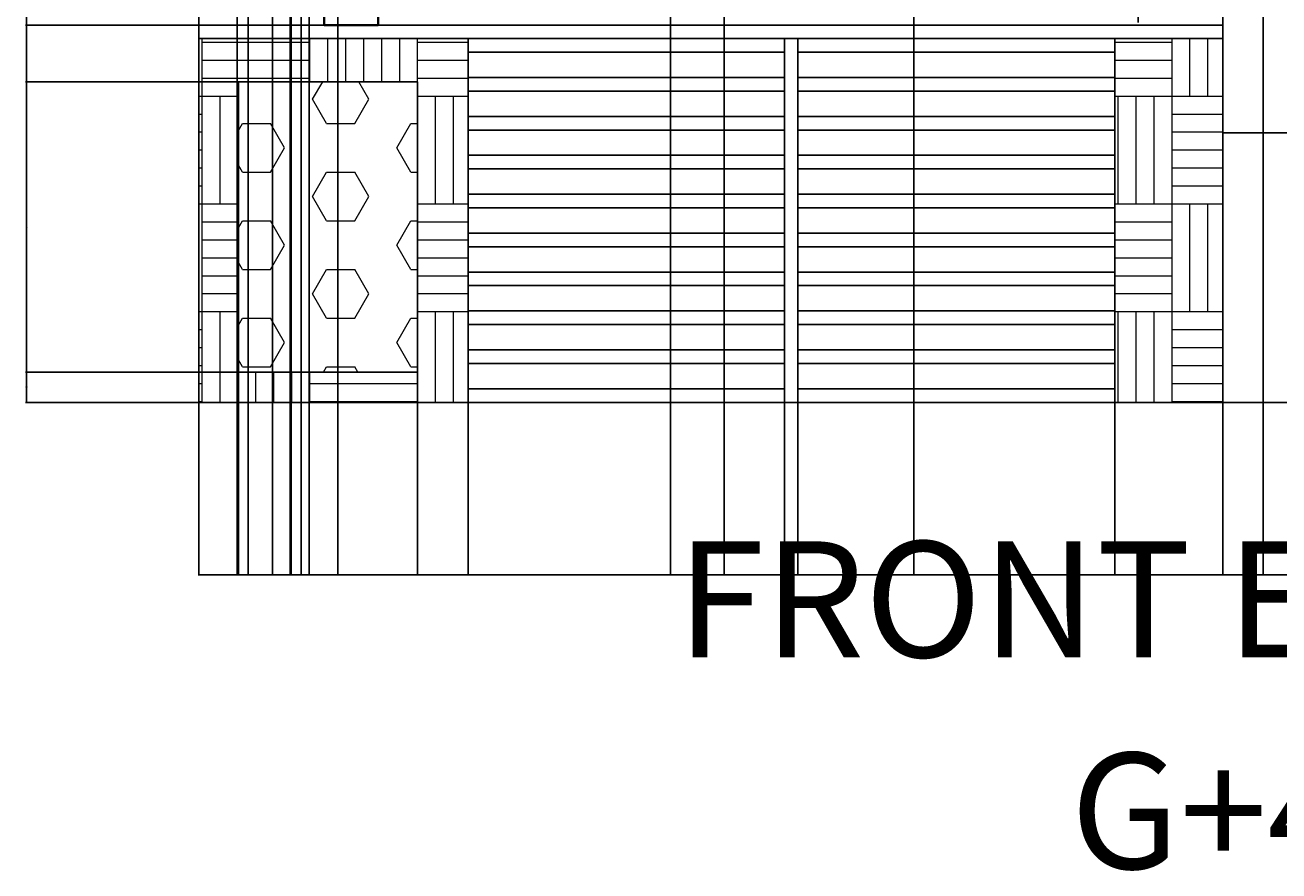
# Model space of a CAD drawing. Units: inches. Extents: x -15 to 605, y -220 to 570.
# Tile 1 of 10: x -15 to 265, y -220 to -32. Entities that reach past the tile are written whole.
import ezdxf

# ---------------------------------------------------------------- set-up
doc = ezdxf.new("R2010")
doc.units = ezdxf.units.IN
doc.header["$MEASUREMENT"] = 0
for name, color, linetype, lineweight in [('A-ANNO-DIMS', 2, 'Continuous', 18), ('A-ANNO-TEXT', 7, 'Continuous', 25), ('A-COLS', 7, 'Continuous', 35), ('A-ELEV-PATT', 8, 'Continuous', 13), ('C-SITE', 3, 'Continuous', 25)]:
    doc.layers.add(name, color=color, linetype=linetype, lineweight=lineweight)
doc.styles.get("Standard").update_dxf_attribs({"font": 'arial.ttf'})
doc.dimstyles.get("Standard").update_dxf_attribs({"dimtxt": 0.18, "dimasz": 0.18, "dimexe": 0.18, "dimexo": 0.0625, "dimgap": 0.09, "dimtad": 0, "dimtih": 1, "dimtoh": 1, "dimdec": 4, "dimzin": 0, "dimdsep": 46, "dimtxsty": 'Standard', "dimcen": 0.09, "dimadec": 0, "dimazin": 0, "dimtfac": 1, "dimtdec": 4, "dimtofl": 0, "dimtmove": 0, "dimatfit": 3, "dimfxl": 1, "dimtolj": 1, "dimtzin": 0, "dimarcsym": 0})

# ---------------------------------------------------------------- blocks, each defined once
blk = doc.blocks.new('*D7')
at = {"layer": 'A-ANNO-DIMS', "color": 0, "lineweight": -2, "transparency": 16777216}
for p, q in [((23.99, 3.76), (23.99, -154.76)), ((566.72, -116.24), (566.72, -154.76)), ((24.17, -154.58), (294.96, -154.58)), ((566.54, -154.58), (295.75, -154.58))]:
    blk.add_line(p, q, dxfattribs=at)
at = {"layer": 'A-ANNO-DIMS', "color": 0, "transparency": 16777216}
for points in [[(24.17, -154.55), (24.17, -154.61), (23.99, -154.58)], [(566.54, -154.55), (566.54, -154.61), (566.72, -154.58)]]:
    blk.add_solid(points, dxfattribs=at)
at = {"layer": 'Defpoints', "color": 0, "transparency": 16777216}
for p in [(23.99, 3.82), (566.72, -116.18), (566.72, -154.58)]:
    blk.add_point(p, dxfattribs=at)
at = {"layer": 'A-ANNO-DIMS', "color": 0, "transparency": 16777216, "insert": (295.35, -154.58), "char_height": 0.18, "attachment_point": 5}
blk.add_mtext('\\A1;542.7', dxfattribs=at)
blk = doc.blocks.new('*D9')
at = {"layer": 'A-ANNO-DIMS', "color": 0, "lineweight": -2, "transparency": 16777216}
for p, q in [((503.92, 531.82), (-14.59, 531.82)), ((-14.41, 531.64), (-14.41, 208)), ((-14.41, -116), (-14.41, 207.64)), ((23.92, -116.18), (-14.59, -116.18))]:
    blk.add_line(p, q, dxfattribs=at)
at = {"layer": 'A-ANNO-DIMS', "color": 0, "transparency": 16777216}
for points in [[(-14.44, 531.64), (-14.38, 531.64), (-14.41, 531.82)], [(-14.44, -116), (-14.38, -116), (-14.41, -116.18)]]:
    blk.add_solid(points, dxfattribs=at)
at = {"layer": 'Defpoints', "color": 0, "transparency": 16777216}
for p in [(-14.41, 531.82), (503.99, 531.82), (23.99, -116.18)]:
    blk.add_point(p, dxfattribs=at)
at = {"layer": 'A-ANNO-DIMS', "color": 0, "transparency": 16777216, "insert": (-14.41, 207.82), "char_height": 0.18, "attachment_point": 5}
blk.add_mtext('\\A1;648', dxfattribs=at)
blk = doc.blocks.new('*D23')
at = {"layer": 'A-ANNO-DIMS', "color": 0, "lineweight": -2, "transparency": 16777216}
for p, q in [((54.93, 15.76), (54.93, -154.76)), ((23.99, 3.76), (23.99, -154.76)), ((24.17, -154.58), (39, -154.58)), ((54.75, -154.58), (39.92, -154.58))]:
    blk.add_line(p, q, dxfattribs=at)
at = {"layer": 'A-ANNO-DIMS', "color": 0, "transparency": 16777216}
for points in [[(24.17, -154.55), (24.17, -154.61), (23.99, -154.58)], [(54.75, -154.55), (54.75, -154.61), (54.93, -154.58)]]:
    blk.add_solid(points, dxfattribs=at)
at = {"layer": 'Defpoints', "color": 0, "transparency": 16777216}
for p in [(54.93, 15.82), (23.99, 3.82), (54.93, -154.58)]:
    blk.add_point(p, dxfattribs=at)
at = {"layer": 'A-ANNO-DIMS', "color": 0, "transparency": 16777216, "insert": (39.46, -154.58), "char_height": 0.18, "attachment_point": 5}
blk.add_mtext('\\A1;30.946', dxfattribs=at)
blk = doc.blocks.new('*D24')
at = {"layer": 'A-ANNO-DIMS', "color": 0, "lineweight": -2, "transparency": 16777216}
for p, q in [((54.93, 15.76), (54.93, -154.76)), ((128.99, 15.76), (128.99, -154.76)), ((55.11, -154.58), (91.57, -154.58)), ((128.81, -154.58), (92.35, -154.58))]:
    blk.add_line(p, q, dxfattribs=at)
at = {"layer": 'A-ANNO-DIMS', "color": 0, "transparency": 16777216}
for points in [[(55.11, -154.55), (55.11, -154.61), (54.93, -154.58)], [(128.81, -154.55), (128.81, -154.61), (128.99, -154.58)]]:
    blk.add_solid(points, dxfattribs=at)
at = {"layer": 'Defpoints', "color": 0, "transparency": 16777216}
for p in [(54.93, 15.82), (128.99, 15.82), (128.99, -154.58)]:
    blk.add_point(p, dxfattribs=at)
at = {"layer": 'A-ANNO-DIMS', "color": 0, "transparency": 16777216, "insert": (91.96, -154.58), "char_height": 0.18, "attachment_point": 5}
blk.add_mtext('\\A1;74.05', dxfattribs=at)
blk = doc.blocks.new('*D25')
at = {"layer": 'A-ANNO-DIMS', "color": 0, "lineweight": -2, "transparency": 16777216}
for p, q in [((128.99, 15.76), (128.99, -154.76)), ((140.99, 15.76), (140.99, -154.76)), ((129.17, -154.58), (134.78, -154.58)), ((140.81, -154.58), (135.2, -154.58))]:
    blk.add_line(p, q, dxfattribs=at)
at = {"layer": 'A-ANNO-DIMS', "color": 0, "transparency": 16777216}
for points in [[(129.17, -154.55), (129.17, -154.61), (128.99, -154.58)], [(140.81, -154.55), (140.81, -154.61), (140.99, -154.58)]]:
    blk.add_solid(points, dxfattribs=at)
at = {"layer": 'Defpoints', "color": 0, "transparency": 16777216}
for p in [(128.99, 15.82), (140.99, 15.82), (140.99, -154.58)]:
    blk.add_point(p, dxfattribs=at)
at = {"layer": 'A-ANNO-DIMS', "color": 0, "transparency": 16777216, "insert": (134.99, -154.58), "char_height": 0.18, "attachment_point": 5}
blk.add_mtext('\\A1;12', dxfattribs=at)
blk = doc.blocks.new('*D26')
at = {"layer": 'A-ANNO-DIMS', "color": 0, "lineweight": -2, "transparency": 16777216}
for p, q in [((140.99, 15.76), (140.99, -154.76)), ((183.17, 15.76), (183.17, -154.76)), ((141.17, -154.58), (161.68, -154.58)), ((182.99, -154.58), (162.48, -154.58))]:
    blk.add_line(p, q, dxfattribs=at)
at = {"layer": 'A-ANNO-DIMS', "color": 0, "transparency": 16777216}
for points in [[(141.17, -154.55), (141.17, -154.61), (140.99, -154.58)], [(182.99, -154.55), (182.99, -154.61), (183.17, -154.58)]]:
    blk.add_solid(points, dxfattribs=at)
at = {"layer": 'Defpoints', "color": 0, "transparency": 16777216}
for p in [(140.99, 15.82), (183.17, 15.82), (183.17, -154.58)]:
    blk.add_point(p, dxfattribs=at)
at = {"layer": 'A-ANNO-DIMS', "color": 0, "transparency": 16777216, "insert": (162.08, -154.58), "char_height": 0.18, "attachment_point": 5}
blk.add_mtext('\\A1;42.18', dxfattribs=at)
blk = doc.blocks.new('*D27')
at = {"layer": 'A-ANNO-DIMS', "color": 0, "lineweight": -2, "transparency": 16777216}
for p, q in [((183.17, 15.76), (183.17, -154.76)), ((260.99, 15.76), (260.99, -154.76)), ((183.35, -154.58), (221.69, -154.58)), ((260.81, -154.58), (222.47, -154.58))]:
    blk.add_line(p, q, dxfattribs=at)
at = {"layer": 'A-ANNO-DIMS', "color": 0, "transparency": 16777216}
for points in [[(183.35, -154.55), (183.35, -154.61), (183.17, -154.58)], [(260.81, -154.55), (260.81, -154.61), (260.99, -154.58)]]:
    blk.add_solid(points, dxfattribs=at)
at = {"layer": 'Defpoints', "color": 0, "transparency": 16777216}
for p in [(183.17, 15.82), (260.99, 15.82), (260.99, -154.58)]:
    blk.add_point(p, dxfattribs=at)
at = {"layer": 'A-ANNO-DIMS', "color": 0, "transparency": 16777216, "insert": (222.08, -154.58), "char_height": 0.18, "attachment_point": 5}
blk.add_mtext('\\A1;77.82', dxfattribs=at)
blk = doc.blocks.new('*D28')
at = {"layer": 'A-ANNO-DIMS', "color": 0, "lineweight": -2, "transparency": 16777216}
for p, q in [((260.99, 15.76), (260.99, -154.76)), ((272.99, 15.76), (272.99, -154.76)), ((261.17, -154.58), (266.78, -154.58)), ((272.81, -154.58), (267.2, -154.58))]:
    blk.add_line(p, q, dxfattribs=at)
at = {"layer": 'A-ANNO-DIMS', "color": 0, "transparency": 16777216}
for points in [[(261.17, -154.55), (261.17, -154.61), (260.99, -154.58)], [(272.81, -154.55), (272.81, -154.61), (272.99, -154.58)]]:
    blk.add_solid(points, dxfattribs=at)
at = {"layer": 'Defpoints', "color": 0, "transparency": 16777216}
for p in [(260.99, 15.82), (272.99, 15.82), (272.99, -154.58)]:
    blk.add_point(p, dxfattribs=at)
at = {"layer": 'A-ANNO-DIMS', "color": 0, "transparency": 16777216, "insert": (266.99, -154.58), "char_height": 0.18, "attachment_point": 5}
blk.add_mtext('\\A1;12', dxfattribs=at)
blk = doc.blocks.new('*D39')
at = {"layer": 'A-ANNO-DIMS', "color": 0, "lineweight": -2, "transparency": 16777216}
for p, q in [((32.79, -109.51), (32.79, -154.76)), ((23.99, -116.24), (23.99, -154.76)), ((24.17, -154.58), (28.01, -154.58)), ((32.61, -154.58), (28.76, -154.58))]:
    blk.add_line(p, q, dxfattribs=at)
at = {"layer": 'A-ANNO-DIMS', "color": 0, "transparency": 16777216}
for points in [[(24.17, -154.55), (24.17, -154.61), (23.99, -154.58)], [(32.61, -154.55), (32.61, -154.61), (32.79, -154.58)]]:
    blk.add_solid(points, dxfattribs=at)
at = {"layer": 'Defpoints', "color": 0, "transparency": 16777216}
for p in [(32.79, -109.45), (23.99, -116.18), (32.79, -154.58)]:
    blk.add_point(p, dxfattribs=at)
at = {"layer": 'A-ANNO-DIMS', "color": 0, "transparency": 16777216, "insert": (28.39, -154.58), "char_height": 0.18, "attachment_point": 5}
blk.add_mtext('\\A1;8.801', dxfattribs=at)
blk = doc.blocks.new('*D40')
at = {"layer": 'A-ANNO-DIMS', "color": 0, "lineweight": -2, "transparency": 16777216}
for p, q in [((32.79, -109.51), (32.79, -154.76)), ((72.68, -109.51), (72.68, -154.76)), ((32.97, -154.58), (52.27, -154.58)), ((72.5, -154.58), (53.2, -154.58))]:
    blk.add_line(p, q, dxfattribs=at)
at = {"layer": 'A-ANNO-DIMS', "color": 0, "transparency": 16777216}
for points in [[(32.97, -154.55), (32.97, -154.61), (32.79, -154.58)], [(72.5, -154.55), (72.5, -154.61), (72.68, -154.58)]]:
    blk.add_solid(points, dxfattribs=at)
at = {"layer": 'Defpoints', "color": 0, "transparency": 16777216}
for p in [(32.79, -109.45), (72.68, -109.45), (72.68, -154.58)]:
    blk.add_point(p, dxfattribs=at)
at = {"layer": 'A-ANNO-DIMS', "color": 0, "transparency": 16777216, "insert": (52.74, -154.58), "char_height": 0.18, "attachment_point": 5}
blk.add_mtext('\\A1;39.895', dxfattribs=at)
blk = doc.blocks.new('*D41')
at = {"layer": 'A-ANNO-DIMS', "color": 0, "lineweight": -2, "transparency": 16777216}
for p, q in [((72.68, -109.51), (72.68, -154.76)), ((83.99, -116.24), (83.99, -154.76)), ((72.86, -154.58), (77.88, -154.58)), ((83.81, -154.58), (78.79, -154.58))]:
    blk.add_line(p, q, dxfattribs=at)
at = {"layer": 'A-ANNO-DIMS', "color": 0, "transparency": 16777216}
for points in [[(72.86, -154.55), (72.86, -154.61), (72.68, -154.58)], [(83.81, -154.55), (83.81, -154.61), (83.99, -154.58)]]:
    blk.add_solid(points, dxfattribs=at)
at = {"layer": 'Defpoints', "color": 0, "transparency": 16777216}
for p in [(72.68, -109.45), (83.99, -116.18), (83.99, -154.58)]:
    blk.add_point(p, dxfattribs=at)
at = {"layer": 'A-ANNO-DIMS', "color": 0, "transparency": 16777216, "insert": (78.34, -154.58), "char_height": 0.18, "attachment_point": 5}
blk.add_mtext('\\A1;11.303', dxfattribs=at)
blk = doc.blocks.new('*D42')
at = {"layer": 'A-ANNO-DIMS', "color": 0, "lineweight": -2, "transparency": 16777216}
for p, q in [((83.99, -116.24), (83.99, -154.76)), ((154.43, -116.24), (154.43, -154.76)), ((84.17, -154.58), (118.82, -154.58)), ((154.25, -154.58), (119.6, -154.58))]:
    blk.add_line(p, q, dxfattribs=at)
at = {"layer": 'A-ANNO-DIMS', "color": 0, "transparency": 16777216}
for points in [[(84.17, -154.55), (84.17, -154.61), (83.99, -154.58)], [(154.25, -154.55), (154.25, -154.61), (154.43, -154.58)]]:
    blk.add_solid(points, dxfattribs=at)
at = {"layer": 'Defpoints', "color": 0, "transparency": 16777216}
for p in [(83.99, -116.18), (154.43, -116.18), (154.43, -154.58)]:
    blk.add_point(p, dxfattribs=at)
at = {"layer": 'A-ANNO-DIMS', "color": 0, "transparency": 16777216, "insert": (119.21, -154.58), "char_height": 0.18, "attachment_point": 5}
blk.add_mtext('\\A1;70.45', dxfattribs=at)
blk = doc.blocks.new('*D43')
at = {"layer": 'A-ANNO-DIMS', "color": 0, "lineweight": -2, "transparency": 16777216}
for p, q in [((154.43, -116.24), (154.43, -154.76)), ((157.4, -116.24), (157.4, -154.76)), ((154.61, -154.58), (155.52, -154.58)), ((157.22, -154.58), (156.31, -154.58))]:
    blk.add_line(p, q, dxfattribs=at)
at = {"layer": 'A-ANNO-DIMS', "color": 0, "transparency": 16777216}
for points in [[(154.61, -154.55), (154.61, -154.61), (154.43, -154.58)], [(157.22, -154.55), (157.22, -154.61), (157.4, -154.58)]]:
    blk.add_solid(points, dxfattribs=at)
at = {"layer": 'Defpoints', "color": 0, "transparency": 16777216}
for p in [(154.43, -116.18), (157.4, -116.18), (157.4, -154.58)]:
    blk.add_point(p, dxfattribs=at)
at = {"layer": 'A-ANNO-DIMS', "color": 0, "transparency": 16777216, "insert": (155.92, -154.58), "char_height": 0.18, "attachment_point": 5}
blk.add_mtext('\\A1;2.969', dxfattribs=at)
blk = doc.blocks.new('*D44')
at = {"layer": 'A-ANNO-DIMS', "color": 0, "lineweight": -2, "transparency": 16777216}
for p, q in [((157.4, -116.24), (157.4, -154.76)), ((227.99, -116.24), (227.99, -154.76)), ((157.58, -154.58), (192.3, -154.58)), ((227.81, -154.58), (193.09, -154.58))]:
    blk.add_line(p, q, dxfattribs=at)
at = {"layer": 'A-ANNO-DIMS', "color": 0, "transparency": 16777216}
for points in [[(157.58, -154.55), (157.58, -154.61), (157.4, -154.58)], [(227.81, -154.55), (227.81, -154.61), (227.99, -154.58)]]:
    blk.add_solid(points, dxfattribs=at)
at = {"layer": 'Defpoints', "color": 0, "transparency": 16777216}
for p in [(157.4, -116.18), (227.99, -116.18), (227.99, -154.58)]:
    blk.add_point(p, dxfattribs=at)
at = {"layer": 'A-ANNO-DIMS', "color": 0, "transparency": 16777216, "insert": (192.69, -154.58), "char_height": 0.18, "attachment_point": 5}
blk.add_mtext('\\A1;70.59', dxfattribs=at)
blk = doc.blocks.new('*D45')
at = {"layer": 'A-ANNO-DIMS', "color": 0, "lineweight": -2, "transparency": 16777216}
for p, q in [((227.99, -116.24), (227.99, -154.76)), ((251.99, -116.24), (251.99, -154.76)), ((228.17, -154.58), (239.77, -154.58)), ((251.81, -154.58), (240.21, -154.58))]:
    blk.add_line(p, q, dxfattribs=at)
at = {"layer": 'A-ANNO-DIMS', "color": 0, "transparency": 16777216}
for points in [[(228.17, -154.55), (228.17, -154.61), (227.99, -154.58)], [(251.81, -154.55), (251.81, -154.61), (251.99, -154.58)]]:
    blk.add_solid(points, dxfattribs=at)
at = {"layer": 'Defpoints', "color": 0, "transparency": 16777216}
for p in [(227.99, -116.18), (251.99, -116.18), (251.99, -154.58)]:
    blk.add_point(p, dxfattribs=at)
at = {"layer": 'A-ANNO-DIMS', "color": 0, "transparency": 16777216, "insert": (239.99, -154.58), "char_height": 0.18, "attachment_point": 5}
blk.add_mtext('\\A1;24', dxfattribs=at)
blk = doc.blocks.new('*D46')
at = {"layer": 'A-ANNO-DIMS', "color": 0, "lineweight": -2, "transparency": 16777216}
for p, q in [((251.99, -116.24), (251.99, -154.76)), ((330.43, -116.24), (330.43, -154.76)), ((252.17, -154.58), (290.82, -154.58)), ((330.25, -154.58), (291.6, -154.58))]:
    blk.add_line(p, q, dxfattribs=at)
at = {"layer": 'A-ANNO-DIMS', "color": 0, "transparency": 16777216}
for points in [[(252.17, -154.55), (252.17, -154.61), (251.99, -154.58)], [(330.25, -154.55), (330.25, -154.61), (330.43, -154.58)]]:
    blk.add_solid(points, dxfattribs=at)
at = {"layer": 'Defpoints', "color": 0, "transparency": 16777216}
for p in [(251.99, -116.18), (330.43, -116.18), (330.43, -154.58)]:
    blk.add_point(p, dxfattribs=at)
at = {"layer": 'A-ANNO-DIMS', "color": 0, "transparency": 16777216, "insert": (291.21, -154.58), "char_height": 0.18, "attachment_point": 5}
blk.add_mtext('\\A1;78.45', dxfattribs=at)
blk = doc.blocks.new('*D56')
at = {"layer": 'A-ANNO-DIMS', "color": 0, "lineweight": -2, "transparency": 16777216}
for p, q in [((233.14, -31.58), (233.14, 570.4)), ((233.32, 570.22), (298.47, 570.22)), ((364.53, 570.22), (299.38, 570.22)), ((364.71, -56.12), (364.71, 570.4))]:
    blk.add_line(p, q, dxfattribs=at)
at = {"layer": 'A-ANNO-DIMS', "color": 0, "transparency": 16777216}
for points in [[(233.32, 570.25), (233.32, 570.19), (233.14, 570.22)], [(364.53, 570.25), (364.53, 570.19), (364.71, 570.22)]]:
    blk.add_solid(points, dxfattribs=at)
at = {"layer": 'Defpoints', "color": 0, "transparency": 16777216}
for p in [(364.71, 570.22), (233.14, -31.64), (364.71, -56.18)]:
    blk.add_point(p, dxfattribs=at)
at = {"layer": 'A-ANNO-DIMS', "color": 0, "transparency": 16777216, "insert": (298.93, 570.22), "char_height": 0.18, "attachment_point": 5}
blk.add_mtext('\\A1;131.56', dxfattribs=at)
blk = doc.blocks.new('*D64')
at = {"layer": 'A-ANNO-DIMS', "color": 0, "lineweight": -2, "transparency": 16777216}
for p, q in [((23.92, -32.18), (-14.59, -32.18)), ((-14.41, -32.36), (-14.41, -74)), ((-14.41, -116), (-14.41, -74.36)), ((23.92, -116.18), (-14.59, -116.18))]:
    blk.add_line(p, q, dxfattribs=at)
at = {"layer": 'A-ANNO-DIMS', "color": 0, "transparency": 16777216}
for points in [[(-14.44, -32.36), (-14.38, -32.36), (-14.41, -32.18)], [(-14.44, -116), (-14.38, -116), (-14.41, -116.18)]]:
    blk.add_solid(points, dxfattribs=at)
at = {"layer": 'Defpoints', "color": 0, "transparency": 16777216}
for p in [(-14.41, -32.18), (23.99, -32.18), (23.99, -116.18)]:
    blk.add_point(p, dxfattribs=at)
at = {"layer": 'A-ANNO-DIMS', "color": 0, "transparency": 16777216, "insert": (-14.41, -74.18), "char_height": 0.18, "attachment_point": 5}
blk.add_mtext('\\A1;84', dxfattribs=at)
blk = doc.blocks.new('*D65')
at = {"layer": 'A-ANNO-DIMS', "color": 0, "lineweight": -2, "transparency": 16777216}
for p, q in [((32.73, -109.45), (-14.59, -109.45)), ((-14.41, -109.63), (-14.41, -112.63)), ((-14.41, -116), (-14.41, -113)), ((23.92, -116.18), (-14.59, -116.18))]:
    blk.add_line(p, q, dxfattribs=at)
at = {"layer": 'A-ANNO-DIMS', "color": 0, "transparency": 16777216}
for points in [[(-14.44, -109.63), (-14.38, -109.63), (-14.41, -109.45)], [(-14.44, -116), (-14.38, -116), (-14.41, -116.18)]]:
    blk.add_solid(points, dxfattribs=at)
at = {"layer": 'Defpoints', "color": 0, "transparency": 16777216}
for p in [(-14.41, -109.45), (32.79, -109.45), (23.99, -116.18)]:
    blk.add_point(p, dxfattribs=at)
at = {"layer": 'A-ANNO-DIMS', "color": 0, "transparency": 16777216, "insert": (-14.41, -112.81), "char_height": 0.18, "attachment_point": 5}
blk.add_mtext('\\A1;6.733', dxfattribs=at)
blk = doc.blocks.new('*D66')
at = {"layer": 'A-ANNO-DIMS', "color": 0, "lineweight": -2, "transparency": 16777216}
for p, q in [((32.73, -44.82), (-14.59, -44.82)), ((-14.41, -45), (-14.41, -76.95)), ((-14.41, -109.27), (-14.41, -77.32)), ((32.73, -109.45), (-14.59, -109.45))]:
    blk.add_line(p, q, dxfattribs=at)
at = {"layer": 'A-ANNO-DIMS', "color": 0, "transparency": 16777216}
for points in [[(-14.44, -45), (-14.38, -45), (-14.41, -44.82)], [(-14.44, -109.27), (-14.38, -109.27), (-14.41, -109.45)]]:
    blk.add_solid(points, dxfattribs=at)
at = {"layer": 'Defpoints', "color": 0, "transparency": 16777216}
for p in [(-14.41, -44.82), (32.79, -44.82), (32.79, -109.45)]:
    blk.add_point(p, dxfattribs=at)
at = {"layer": 'A-ANNO-DIMS', "color": 0, "transparency": 16777216, "insert": (-14.41, -77.14), "char_height": 0.18, "attachment_point": 5}
blk.add_mtext('\\A1;64.62', dxfattribs=at)
blk = doc.blocks.new('*D68')
at = {"layer": 'A-ANNO-DIMS', "color": 0, "lineweight": -2, "transparency": 16777216}
for p, q in [((252.05, -56.18), (605.3, -56.18)), ((605.12, -56.36), (605.12, -86)), ((605.12, -116), (605.12, -86.36)), ((252.05, -116.18), (605.3, -116.18))]:
    blk.add_line(p, q, dxfattribs=at)
at = {"layer": 'A-ANNO-DIMS', "color": 0, "transparency": 16777216}
for points in [[(605.09, -56.36), (605.15, -56.36), (605.12, -56.18)], [(605.09, -116), (605.15, -116), (605.12, -116.18)]]:
    blk.add_solid(points, dxfattribs=at)
at = {"layer": 'Defpoints', "color": 0, "transparency": 16777216}
for p in [(251.99, -56.18), (605.12, -56.18), (251.99, -116.18)]:
    blk.add_point(p, dxfattribs=at)
at = {"layer": 'A-ANNO-DIMS', "color": 0, "transparency": 16777216, "insert": (605.12, -86.18), "char_height": 0.18, "attachment_point": 5}
blk.add_mtext('\\A1;60', dxfattribs=at)
blk = doc.blocks.new('*D104')
at = {"layer": 'A-ANNO-DIMS', "color": 0, "lineweight": -2, "transparency": 16777216}
for p, q in [((251.99, -56.12), (251.99, 570.4)), ((252.17, 570.22), (267.39, 570.22)), ((283.41, 570.22), (268.18, 570.22)), ((283.59, -84.79), (283.59, 570.4))]:
    blk.add_line(p, q, dxfattribs=at)
at = {"layer": 'A-ANNO-DIMS', "color": 0, "transparency": 16777216}
for points in [[(252.17, 570.25), (252.17, 570.19), (251.99, 570.22)], [(283.41, 570.25), (283.41, 570.19), (283.59, 570.22)]]:
    blk.add_solid(points, dxfattribs=at)
at = {"layer": 'Defpoints', "color": 0, "transparency": 16777216}
for p in [(283.59, 570.22), (251.99, -56.18), (283.59, -84.86)]:
    blk.add_point(p, dxfattribs=at)
at = {"layer": 'A-ANNO-DIMS', "color": 0, "transparency": 16777216, "insert": (267.79, 570.22), "char_height": 0.18, "attachment_point": 5}
blk.add_mtext('\\A1;31.60', dxfattribs=at)
blk = doc.blocks.new('*D111')
at = {"layer": 'A-ANNO-DIMS', "color": 0, "lineweight": -2, "transparency": 16777216}
for p, q in [((32.53, 12.22), (32.53, -154.76)), ((34.93, 12.22), (34.93, -154.76)), ((32.71, -154.58), (33.41, -154.58)), ((34.75, -154.58), (34.06, -154.58))]:
    blk.add_line(p, q, dxfattribs=at)
at = {"layer": 'A-ANNO-DIMS', "color": 0, "transparency": 16777216}
for points in [[(32.71, -154.55), (32.71, -154.61), (32.53, -154.58)], [(34.75, -154.55), (34.75, -154.61), (34.93, -154.58)]]:
    blk.add_solid(points, dxfattribs=at)
at = {"layer": 'Defpoints', "color": 0, "transparency": 16777216}
for p in [(32.53, 12.28), (34.93, 12.28), (34.93, -154.58)]:
    blk.add_point(p, dxfattribs=at)
at = {"layer": 'A-ANNO-DIMS', "color": 0, "transparency": 16777216, "insert": (33.73, -154.58), "char_height": 0.18, "attachment_point": 5}
blk.add_mtext('\\A1;2.40', dxfattribs=at)
blk = doc.blocks.new('*D112')
at = {"layer": 'A-ANNO-DIMS', "color": 0, "lineweight": -2, "transparency": 16777216}
for p, q in [((44.53, 12.22), (44.53, -154.76)), ((48.53, 12.22), (48.53, -154.76)), ((44.71, -154.58), (46.21, -154.58)), ((48.35, -154.58), (46.86, -154.58))]:
    blk.add_line(p, q, dxfattribs=at)
at = {"layer": 'A-ANNO-DIMS', "color": 0, "transparency": 16777216}
for points in [[(44.71, -154.55), (44.71, -154.61), (44.53, -154.58)], [(48.35, -154.55), (48.35, -154.61), (48.53, -154.58)]]:
    blk.add_solid(points, dxfattribs=at)
at = {"layer": 'Defpoints', "color": 0, "transparency": 16777216}
for p in [(44.53, 12.28), (48.53, 12.28), (48.53, -154.58)]:
    blk.add_point(p, dxfattribs=at)
at = {"layer": 'A-ANNO-DIMS', "color": 0, "transparency": 16777216, "insert": (46.53, -154.58), "char_height": 0.18, "attachment_point": 5}
blk.add_mtext('\\A1;4.00', dxfattribs=at)
blk = doc.blocks.new('*D113')
at = {"layer": 'A-ANNO-DIMS', "color": 0, "lineweight": -2, "transparency": 16777216}
for p, q in [((44.35, 231.76), (44.35, -154.76)), ((46.75, 231.76), (46.75, -154.76)), ((44.53, -154.58), (45.23, -154.58)), ((46.57, -154.58), (45.88, -154.58))]:
    blk.add_line(p, q, dxfattribs=at)
at = {"layer": 'A-ANNO-DIMS', "color": 0, "transparency": 16777216}
for points in [[(44.53, -154.55), (44.53, -154.61), (44.35, -154.58)], [(46.57, -154.55), (46.57, -154.61), (46.75, -154.58)]]:
    blk.add_solid(points, dxfattribs=at)
at = {"layer": 'Defpoints', "color": 0, "transparency": 16777216}
for p in [(44.35, 231.82), (46.75, 231.82), (46.75, -154.58)]:
    blk.add_point(p, dxfattribs=at)
at = {"layer": 'A-ANNO-DIMS', "color": 0, "transparency": 16777216, "insert": (45.55, -154.58), "char_height": 0.18, "attachment_point": 5}
blk.add_mtext('\\A1;2.40', dxfattribs=at)
blk = doc.blocks.new('*D114')
at = {"layer": 'A-ANNO-DIMS', "color": 0, "lineweight": -2, "transparency": 16777216}
for p, q in [((40.35, 231.76), (40.35, -154.76)), ((44.35, 231.76), (44.35, -154.76)), ((40.53, -154.58), (42.03, -154.58)), ((44.17, -154.58), (42.68, -154.58))]:
    blk.add_line(p, q, dxfattribs=at)
at = {"layer": 'A-ANNO-DIMS', "color": 0, "transparency": 16777216}
for points in [[(40.53, -154.55), (40.53, -154.61), (40.35, -154.58)], [(44.17, -154.55), (44.17, -154.61), (44.35, -154.58)]]:
    blk.add_solid(points, dxfattribs=at)
at = {"layer": 'Defpoints', "color": 0, "transparency": 16777216}
for p in [(40.35, 231.82), (44.35, 231.82), (44.35, -154.58)]:
    blk.add_point(p, dxfattribs=at)
at = {"layer": 'A-ANNO-DIMS', "color": 0, "transparency": 16777216, "insert": (42.35, -154.58), "char_height": 0.18, "attachment_point": 5}
blk.add_mtext('\\A1;4.00', dxfattribs=at)

msp = doc.modelspace()

# ---------------------------------------------------------------- hatches: boundary and pattern name
at = {"layer": 'A-ELEV-PATT'}
h = msp.add_hatch(dxfattribs=at)
h.set_pattern_fill('AR-PARQ1', color=256, scale=2)
h.set_pattern_definition([(90, (-191.319, 0), (-24, 24), [24, -24]), (90, (-187.319, 0), (-24, 24), [24, -24]), (90, (-183.319, 0), (-24, 24), [24, -24]), (90, (-179.319, 0), (-24, 24), [24, -24]), (90, (-175.319, 0), (-24, 24), [24, -24]), (90, (-171.319, 0), (-24, 24), [24, -24]), (90, (-167.319, 0), (-24, 24), [24, -24]), (0, (-191.319, 24), (24, -24), [24, -24]), (0, (-191.319, 28), (24, -24), [24, -24]), (0, (-191.319, 32), (24, -24), [24, -24]), (0, (-191.319, 36), (24, -24), [24, -24]), (0, (-191.319, 40), (24, -24), [24, -24]), (0, (-191.319, 44), (24, -24), [24, -24]), (0, (-191.319, 48), (24, -24), [24, -24])])
h.paths.add_polyline_path([(392.6125, -39.8843), (378.2334, -39.8843), (354.916, -116.1813), (370.8496, -116.1813)])
h.paths.add_polyline_path([(368.1292, -39.8843), (353.7501, -39.8843), (330.4327, -116.1813), (346.3663, -116.1813)])
h.paths.add_polyline_path([(566.7161, -45.9373), (413.9976, -45.9373), (413.9976, -116.1813), (566.7161, -116.1813)])
h.paths.add_polyline_path([(251.9872, -35.1813), (227.9872, -35.1813), (227.9872, -116.1813), (251.9872, -116.1813)])
h.paths.add_polyline_path([(83.9872, -35.1813), (23.9872, -35.1813), (23.9872, -116.1813), (83.9872, -116.1813), (83.9872, -113.1422)])
h.paths.add_polyline_path([(72.6838, -44.8238), (72.6838, -109.4483), (32.7886, -109.4483), (32.7886, -44.8238)], flags=16)
h = msp.add_hatch(dxfattribs=at)
h.set_pattern_fill('HEX', color=256, scale=50)
h.set_pattern_definition([(0, (-191.319, 0), (0, 10.8253), [6.25, -12.5]), (120, (-191.319, 0), (-9.375, -5.41266), [6.25, -12.5]), (60, (-185.069, 0), (-9.375, 5.41266), [6.25, -12.5])])
h.paths.add_polyline_path([(72.6838, -44.8238), (32.7886, -44.8238), (32.7886, -109.4483), (72.6838, -109.4483)])

# ---------------------------------------------------------------- linework, layer by layer
at = {"layer": 'A-COLS'}
msp.add_lwpolyline([(51.9067, 3.8187), (63.9067, 3.8187), (63.9067, -32.1813), (51.9067, -32.1813)], close=True, dxfattribs=at)
at = {"layer": 'C-SITE'}
for p, q in [((23.9872, -32.1813), (251.9872, -32.1813)), ((23.9872, -32.1813), (23.9872, -35.1813)), ((251.9872, -32.1813), (251.9872, -116.1813)), ((23.9872, -35.1813), (251.9872, -35.1813)), ((23.9872, -35.1813), (23.9872, -116.1813)), ((83.9872, -35.1813), (83.9872, -116.1813)), ((154.4326, -35.1813), (154.4326, -116.1813)), ((157.4017, -35.1813), (157.4017, -116.1813)), ((227.9872, -35.1813), (227.9872, -116.1813)), ((251.9872, -56.1813), (348.7695, -56.1813)), ((23.9872, -116.1813), (503.9872, -116.1813))]:
    msp.add_line(p, q, dxfattribs=at)
for points in [[(154.4326, -38.2204), (83.9872, -38.2204), (83.9872, -35.1813), (227.9872, -35.1813), (227.9872, -38.2204), (157.4017, -38.2204)], [(154.4326, -46.8827), (83.9872, -46.8827), (83.9872, -43.8436), (154.4326, -43.8436)], [(157.4017, -43.8436), (227.9872, -43.8436), (227.9872, -46.8827), (157.4017, -46.8827)], [(154.4326, -55.545), (83.9872, -55.545), (83.9872, -52.5059), (154.4326, -52.5059)], [(157.4017, -52.5059), (227.9872, -52.5059), (227.9872, -55.545), (157.4017, -55.545)], [(154.4326, -64.2073), (83.9872, -64.2073), (83.9872, -61.1682), (154.4326, -61.1682)], [(157.4017, -61.1682), (227.9872, -61.1682), (227.9872, -64.2073), (157.4017, -64.2073)], [(154.4326, -72.8697), (83.9872, -72.8697), (83.9872, -69.8306), (154.4326, -69.8306)], [(157.4017, -69.8306), (227.9872, -69.8306), (227.9872, -72.8697), (157.4017, -72.8697)], [(154.4326, -81.532), (83.9872, -81.532), (83.9872, -78.4929), (154.4326, -78.4929)], [(157.4017, -78.4929), (227.9872, -78.4929), (227.9872, -81.532), (157.4017, -81.532)], [(154.4326, -90.1943), (83.9872, -90.1943), (83.9872, -87.1552), (154.4326, -87.1552)], [(157.4017, -87.1552), (227.9872, -87.1552), (227.9872, -90.1943), (157.4017, -90.1943)], [(154.4326, -98.8566), (83.9872, -98.8566), (83.9872, -95.8175), (154.4326, -95.8175)], [(157.4017, -95.8175), (227.9872, -95.8175), (227.9872, -98.8566), (157.4017, -98.8566)], [(154.4326, -107.5189), (83.9872, -107.5189), (83.9872, -104.4799), (154.4326, -104.4799)], [(157.4017, -104.4799), (227.9872, -104.4799), (227.9872, -107.5189), (157.4017, -107.5189)], [(157.4017, -113.1422), (227.9872, -113.1422), (227.9872, -116.1813), (83.9872, -116.1813), (83.9872, -113.1422), (154.4326, -113.1422)]]:
    msp.add_lwpolyline(points, dxfattribs=at)
msp.add_lwpolyline([(32.7886, -44.8238), (72.6838, -44.8238), (72.6838, -109.4483), (32.7886, -109.4483)], close=True, dxfattribs=at)

# ---------------------------------------------------------------- texts
at = {"layer": 'A-ANNO-TEXT'}
for s, height, p in [('FRONT ELEVATION', 25.818282, (130.4215, -172.9392)), ('G+4', 25.81828, (218.0971, -220.0392))]:
    msp.add_text(s, height=height, dxfattribs=at).set_placement(p)

# ---------------------------------------------------------------- dimensions: what is measured, and where the dimension line sits
at = {"layer": 'A-ANNO-DIMS'}
for base, p1, p2, override, picture, middle in [((364.7066, 570.2187), (233.1439, -31.6396), (364.7066, -56.1813), {"dimdec": 2, "dimlfac": 1, "dimrnd": 0, "dimzin": 0, "dimdsep": 46, "dimlunit": 2}, '*D56', (298.9252, 570.2187)), ((283.5871, 570.2187), (251.9872, -56.1813), (283.5871, -84.8572), {"dimdec": 2, "dimlfac": 1, "dimrnd": 0, "dimzin": 0, "dimdsep": 46, "dimlunit": 2}, '*D104', (267.7872, 570.2187)), ((44.3542, -154.5813), (40.354, 231.8187), (44.3542, 231.8187), {"dimdec": 2, "dimlfac": 1, "dimrnd": 0, "dimzin": 0, "dimdsep": 46, "dimlunit": 2}, '*D114', (42.3541, -154.5813)), ((46.7542, -154.5813), (44.3542, 231.8187), (46.7542, 231.8187), {"dimdec": 2, "dimlfac": 1, "dimrnd": 0, "dimzin": 0, "dimdsep": 46, "dimlunit": 2}, '*D113', (45.5542, -154.5813)), ((54.933, -154.5813), (23.9872, 3.8187), (54.933, 15.8187), {"dimdec": 3, "dimlfac": 1, "dimrnd": 0, "dimzin": 0, "dimdsep": 46, "dimlunit": 2}, '*D23', (39.4601, -154.5813)), ((128.9872, -154.5813), (54.933, 15.8187), (128.9872, 15.8187), {"dimdec": 2, "dimlfac": 1, "dimrnd": 0, "dimzin": 0, "dimdsep": 46, "dimlunit": 2}, '*D24', (91.9601, -154.5813)), ((140.9872, -154.5813), (128.9872, 15.8187), (140.9872, 15.8187), {"dimdec": 0, "dimlfac": 1, "dimrnd": 0, "dimzin": 0, "dimdsep": 46, "dimlunit": 2}, '*D25', (134.9872, -154.5813)), ((183.1686, -154.5813), (140.9872, 15.8187), (183.1686, 15.8187), {"dimdec": 2, "dimlfac": 1, "dimrnd": 0, "dimzin": 0, "dimdsep": 46, "dimlunit": 2}, '*D26', (162.0779, -154.5813)), ((260.9872, -154.5813), (183.1686, 15.8187), (260.9872, 15.8187), {"dimdec": 2, "dimlfac": 1, "dimrnd": 0, "dimzin": 0, "dimdsep": 46, "dimlunit": 2}, '*D27', (222.0779, -154.5813)), ((272.9872, -154.5813), (260.9872, 15.8187), (272.9872, 15.8187), {"dimdec": 0, "dimlfac": 1, "dimrnd": 0, "dimzin": 0, "dimdsep": 46, "dimlunit": 2}, '*D28', (266.9872, -154.5813)), ((34.9324, -154.5813), (32.5323, 12.2791), (34.9324, 12.2791), {"dimdec": 2, "dimlfac": 1, "dimrnd": 0, "dimzin": 0, "dimdsep": 46, "dimlunit": 2}, '*D111', (33.7323, -154.5813)), ((48.5328, -154.5813), (44.5327, 12.2791), (48.5328, 12.2791), {"dimdec": 2, "dimlfac": 1, "dimrnd": 0, "dimzin": 0, "dimdsep": 46, "dimlunit": 2}, '*D112', (46.5327, -154.5813)), ((566.7161, -154.5813), (23.9872, 3.8187), (566.7161, -116.1813), {"dimdec": 1, "dimlfac": 1, "dimrnd": 0, "dimzin": 0, "dimdsep": 46, "dimlunit": 2}, '*D7', (295.3517, -154.5813)), ((32.7886, -154.5813), (23.9872, -116.1813), (32.7886, -109.4483), {"dimdec": 3, "dimlfac": 1, "dimrnd": 0, "dimzin": 0, "dimdsep": 46, "dimlunit": 2}, '*D39', (28.3879, -154.5813)), ((72.6838, -154.5813), (32.7886, -109.4483), (72.6838, -109.4483), {"dimdec": 3, "dimlfac": 1, "dimrnd": 0, "dimzin": 0, "dimdsep": 46, "dimlunit": 2}, '*D40', (52.7362, -154.5813)), ((83.9872, -154.5813), (72.6838, -109.4483), (83.9872, -116.1813), {"dimdec": 3, "dimlfac": 1, "dimrnd": 0, "dimzin": 0, "dimdsep": 46, "dimlunit": 2}, '*D41', (78.3355, -154.5813)), ((154.4326, -154.5813), (83.9872, -116.1813), (154.4326, -116.1813), {"dimdec": 2, "dimlfac": 1, "dimrnd": 0, "dimzin": 0, "dimdsep": 46, "dimlunit": 2}, '*D42', (119.2099, -154.5813)), ((157.4017, -154.5813), (154.4326, -116.1813), (157.4017, -116.1813), {"dimdec": 3, "dimlfac": 1, "dimrnd": 0, "dimzin": 0, "dimdsep": 46, "dimlunit": 2}, '*D43', (155.9171, -154.5813)), ((227.9872, -154.5813), (157.4017, -116.1813), (227.9872, -116.1813), {"dimdec": 2, "dimlfac": 1, "dimrnd": 0, "dimzin": 0, "dimdsep": 46, "dimlunit": 2}, '*D44', (192.6944, -154.5813)), ((251.9872, -154.5813), (227.9872, -116.1813), (251.9872, -116.1813), {"dimdec": 0, "dimlfac": 1, "dimrnd": 0, "dimzin": 0, "dimdsep": 46, "dimlunit": 2}, '*D45', (239.9872, -154.5813)), ((330.4327, -154.5813), (251.9872, -116.1813), (330.4327, -116.1813), {"dimdec": 2, "dimlfac": 1, "dimrnd": 0, "dimzin": 0, "dimdsep": 46, "dimlunit": 2}, '*D46', (291.21, -154.5813))]:
    dim = msp.add_linear_dim(base=base, p1=p1, p2=p2, dimstyle='Standard', override=override, dxfattribs=at)
    dim.commit()
    dim.dimension.update_dxf_attribs({"geometry": picture, "text_midpoint": middle})
for base, p1, p2, override, picture, middle in [((-14.4128, 531.8187), (23.9872, -116.1813), (503.9872, 531.8187), {"dimdec": 0, "dimlfac": 1, "dimrnd": 0, "dimzin": 0, "dimdsep": 46, "dimlunit": 2}, '*D9', (-14.4128, 207.8187)), ((-14.4128, -32.1813), (23.9872, -116.1813), (23.9872, -32.1813), {"dimdec": 0, "dimlfac": 1, "dimrnd": 0, "dimzin": 0, "dimdsep": 46, "dimlunit": 2}, '*D64', (-14.4128, -74.1813)), ((-14.4128, -44.8238), (32.7886, -109.4483), (32.7886, -44.8238), {"dimdec": 2, "dimlfac": 1, "dimrnd": 0, "dimzin": 0, "dimdsep": 46, "dimlunit": 2}, '*D66', (-14.4128, -77.136)), ((605.1161, -56.1813), (251.9872, -116.1813), (251.9872, -56.1813), {"dimdec": 0, "dimlfac": 1, "dimrnd": 0, "dimzin": 0, "dimdsep": 46, "dimlunit": 2}, '*D68', (605.1161, -86.1813)), ((-14.4128, -109.4483), (23.9872, -116.1813), (32.7886, -109.4483), {"dimdec": 3, "dimlfac": 1, "dimrnd": 0, "dimzin": 0, "dimdsep": 46, "dimlunit": 2}, '*D65', (-14.4128, -112.8148))]:
    dim = msp.add_linear_dim(base=base, p1=p1, p2=p2, angle=90, dimstyle='Standard', override=override, dxfattribs=at)
    dim.commit()
    dim.dimension.update_dxf_attribs({"geometry": picture, "text_midpoint": middle})

doc.saveas('drawing.dxf')
